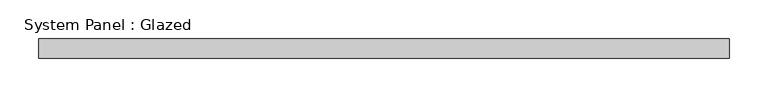
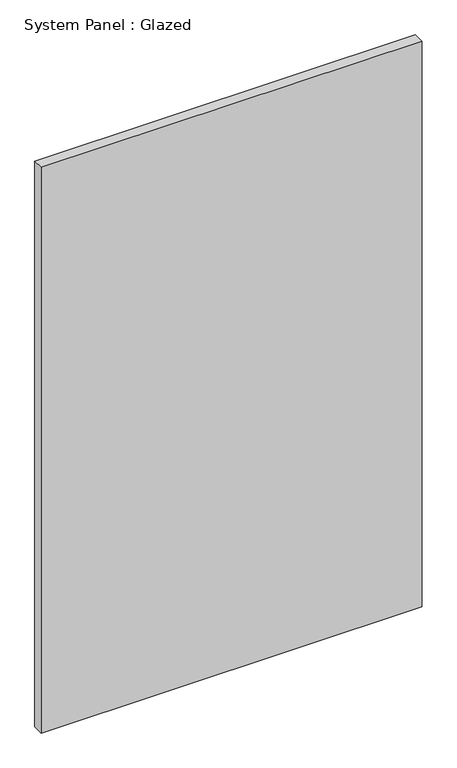
"""IFC4 building model written with IfcOpenShell, lengths in millimetres: plate geometry, System Panel : Glazed."""

from ifc_helpers import new_model, si_unit, origin, origin_with_axes, place, context, project, spatial, polyline, outline, extrude, source, transform, mapped, element, save


def system_panel_glazed_a6d6e80d(model_context):
    return source(origin(), model_context, "Body", "SweptSolid", [
        extrude(outline(polyline([(447.675, 19.05), (-447.675, 19.05), (-447.675, 44.45), (447.675, 44.45), (447.675, 19.05)])), origin_with_axes(), (0.0, 0.0, 1.0), 1405.6819),
    ])


if __name__ == "__main__":
    model = new_model("IFC4")
    model_context = context("Model", 3, world=origin())
    ifc_project = project(units=[si_unit("LENGTHUNIT", "METRE", prefix="MILLI")], contexts=[model_context])
    site = spatial("IfcSite", under=ifc_project)
    building = spatial("IfcBuilding", under=site)
    placement = place(None, origin())
    system_panel_glazed_shape = system_panel_glazed_a6d6e80d(model_context)
    element("IfcPlate", 1, ObjectType="System Panel : Glazed", at=placement, inside=building, context=model_context, shape_type="MappedRepresentation", body=[
        mapped(system_panel_glazed_shape, transform((0.0, 0.0, 0.0), x_axis=(1.0, 0.0, 0.0), y_axis=(0.0, 1.0, 0.0), z_axis=(0.0, 0.0, 1.0))),
    ])
    save(model, "model.ifc")

# Revit data of these elements
# Type "System Panel : Glazed"
#   Construction Type Id = "GSP4R"
#   Analytic Construction = "1/8 in Pilkington single glazing"
#   Visual Light Transmittance = 0.9
#   Solar Heat Gain Coefficient = 0.86
#   Heat Transfer Coefficient (U) = 1.18115 BTU/(h·ft²·°F)
#   Define Thermal Properties by = 1
# Element 1 (IfcPlate, "System Panel : Glazed")
#   Materials on its faces: "Glass"
# Materials
#   "Glass": class "Glass", colour RGB 0 128 192, transparency 0.75, Description = "Soda Lime Glass", Cost = 0
